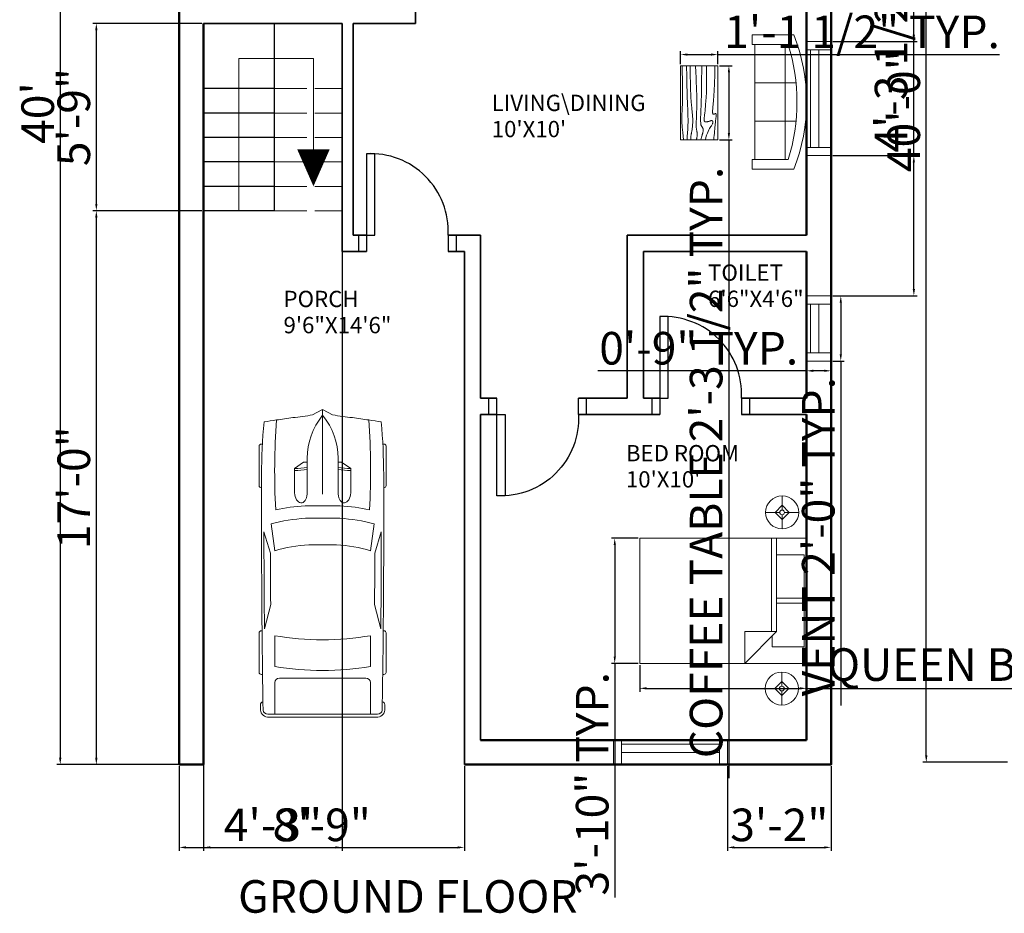
# Model space of a CAD drawing. Units: inches. Extents: x 2296 to 3335, y 495 to 1294.
# Tile 1 of 7: x 2296 to 2659, y 532 to 862. Entities that reach past the tile are written whole.
import ezdxf

# ---------------------------------------------------------------- set-up
doc = ezdxf.new("R2010")
doc.units = ezdxf.units.IN
doc.linetypes.add('ACAD_ISO02W100', pattern=[15, 12, -3])
for name, color, linetype, lineweight in [('A-ANNO-DIMS', 2, 'Continuous', 18), ('A-ANNO-SYMB', 7, 'Continuous', 18), ('A-ANNO-TEXT', 7, 'Continuous', 35), ('A-AREA-IDEN', 7, 'Continuous', 18), ('A-EQPM-VEHL', 8, 'Continuous', 13), ('A-FLOR-STRS', 7, 'Continuous', 25), ('A-FLOR-STRS-OVHD', 7, 'ACAD_ISO02W100', 18), ('DOORS', 1, 'Continuous', 25), ('E-LITE', 2, 'Continuous', 18), ('FURNITURE', 2, 'Continuous', 18), ('INNER WALL', 6, 'Continuous', 35), ('OUTER WALL', 5, 'Continuous', 50), ('VENTILATOR', 4, 'Continuous', 18), ('WINDOWS', 3, 'Continuous', 18)]:
    doc.layers.add(name, color=color, linetype=linetype, lineweight=lineweight)
doc.styles.get("Standard").update_dxf_attribs({"font": 'arial.ttf'})
doc.dimstyles.new('ISO-25', dxfattribs={"dimtxt": 12, "dimasz": 2.5, "dimexe": 1.25, "dimexo": 0.625, "dimtad": 1, "dimdec": 1, "dimlunit": 3, "dimtxsty": 'Standard', "dimcen": 2.5, "dimadec": 0, "dimazin": 0, "dimtfac": 1, "dimtdec": 1, "dimtmove": 0, "dimatfit": 3, "dimfxl": 1, "dimarcsym": 0})

# ---------------------------------------------------------------- blocks, each defined once
blk = doc.blocks.new('*U2')
for p, q in [((21.1, 37.41), (21.1, 36.83)), ((46.55, 38.89), (22.35, 38.89)), ((47.8, 37.39), (47.8, 37.41)), ((135.45, 37.07), (135.45, 37.41)), ((136.7, 38.89), (160.9, 38.89)), ((162.15, 37.41), (162.15, 36.77)), ((70.03, 31.54), (86.41, 29.35)), ((87.99, 31.87), (74.76, 35.92)), ((134.31, 35.6), (119.29, 31.78)), ((186.47, -33.5), (186.47, 33.5)), ((188.4, -32.76), (188.4, 32.76)), ((138.42, 29.35), (157.25, 29.35)), ((164.52, 26.39), (164.52, -26.39)), ((186.47, 29.35), (167.01, 29.35)), ((32.27, 11.63), (36.13, 17.17)), ((36.13, 17.17), (50.94, 17.17)), ((3.27, 6.13), (0.1, 0.41)), ((29.77, 9.51), (51.68, 9.51)), ((32.12, 9.51), (32.12, 11.15)), ((58.92, -10.77), (58.92, 10.77)), ((66.55, -10.53), (66.55, 10.53)), ((82.74, 8.5), (82.74, -8.5)), ((186.47, -10.53), (186.47, 10.53)), ((0, 0), (51.68, 0)), ((0.1, -0.41), (3.27, -6.13)), ((29.77, -9.51), (51.68, -9.51)), ((32.12, -9.51), (32.12, -11.15)), ((32.27, -11.63), (36.13, -17.17)), ((36.13, -17.17), (50.94, -17.17)), ((86.41, -29.35), (70.03, -31.54)), ((157.25, -29.35), (138.42, -29.35)), ((167.01, -29.35), (186.47, -29.35)), ((87.99, -31.87), (74.76, -35.92)), ((134.31, -35.6), (119.29, -31.78)), ((21.1, -37.41), (21.1, -36.83)), ((46.55, -38.89), (22.35, -38.89)), ((47.8, -37.39), (47.8, -37.41)), ((135.45, -37.07), (135.45, -37.41)), ((136.7, -38.89), (160.9, -38.89)), ((162.15, -37.41), (162.15, -36.77))]:
    blk.add_line(p, q)
for centre, major_axis, ratio, start_param, end_param in [((41.19, -490.86), (0, 528.23), 0.842304, 0.00281, 0.075598), ((22.35, 37.41), (0, -1.48), 0.842304, 3.141593, 4.712389), ((64.48, -10555.62), (0, 10593.03), 0.842304, -0.013397, 0.002797), ((46.55, 37.41), (0, 1.48), 0.842304, -1.570796, 0), ((136.7, 37.41), (0, -1.48), 0.842304, 3.141593, 4.712389), ((160.9, 37.41), (0, 1.48), 0.842304, -1.570796, 0), ((180.63, 35.84), (0, 2.22), 0.842304, -0.013017, 1.249894), ((64.48, -10556.36), (0, 10595.31), 0.842304, -0.013397, -0.013017), ((183.98, 33.5), (0, -2.96), 0.842304, 1.570796, 3.128196), ((183.98, 32.76), (0, -5.25), 0.842304, 1.570796, 3.128196), ((266.03, -27.52), (0, 313.31), 0.842304, 1.367076, 1.39176), ((135.29, 5.39), (0, 81.77), 0.842304, 1.245306, 1.50788), ((64.48, -10555.62), (0, -10591.55), 0.842304, 3.133765, 3.140441), ((95.79, -3666.35), (0, -3698.24), 0.842304, 3.134049, 3.144098), ((259.18, -27.52), (0, -305.3), 0.842304, 4.528606, 4.561838), ((37.47, -593.96), (0, -623.33), 0.842304, 3.096046, 3.200911), ((134.4, 5.39), (0, -89.78), 0.842304, 4.449482, 4.652344), ((149.6, 2.8), (0, -79.58), 0.842304, 4.372215, 4.640744), ((17.08, 0), (0, 147.02), 0.842304, 4.511394, 4.913384), ((35.91, 0), (0, 147.02), 0.842304, 4.511394, 4.913384), ((167.01, 26.39), (0, 2.96), 0.842304, 0, 1.570796), ((-204.49, 52.4), (0, -250.96), 0.842304, 1.385369, 1.434372), ((13.04, 17.01), (0, 27.42), 0.842304, 4.435146, 4.718221), ((14.2, 17.01), (0, 27.42), 0.842304, 4.435146, 4.718221), ((50.79, 13.34), (6.34, -0.36), 0.603834, -1.395552, 1.581315), ((29.77, -46.66), (0, 56.17), 0.842304, 0, 0.590319), ((32.75, 11.15), (0, 0.74), 0.842304, 0.879714, 1.570796), ((0.62, 0), (0, -0.74), 0.842304, 4.131459, 5.293319), ((29.77, 46.66), (0, 56.17), 0.842304, 2.551274, 3.141593), ((-204.49, -52.4), (0, 250.96), 0.842304, -1.434372, -1.385369), ((32.75, -11.15), (0, -0.74), 0.842304, 4.712389, 5.403472), ((13.04, -17.01), (0, -27.42), 0.842304, 1.564964, 1.848039), ((14.2, -17.01), (0, -27.42), 0.842304, 1.564964, 1.848039), ((134.4, -5.39), (0, -89.78), 0.842304, -1.510751, -1.307889), ((135.29, -5.39), (0, -81.77), 0.842304, -1.50788, -1.245306), ((149.6, -2.8), (0, -79.58), 0.842304, -1.499151, -1.230623), ((259.18, 27.52), (0, 305.3), 0.842304, 1.721348, 1.754579), ((266.03, 27.52), (0, 313.31), 0.842304, 1.749832, 1.774517), ((37.47, 593.96), (0, -623.33), 0.842304, -0.059319, 0.045547), ((167.01, -26.39), (0, -2.96), 0.842304, 4.712389, 6.283185), ((41.19, 490.86), (0, -528.23), 0.842304, -0.075598, -0.00281), ((64.48, 10555.62), (0, -10591.55), 0.842304, 0.001152, 0.007828), ((95.79, 3666.35), (0, -3698.24), 0.842304, -0.002505, 0.007544), ((183.98, -33.5), (0, 2.96), 0.842304, 3.15499, 4.712389), ((183.98, -32.76), (0, -5.25), 0.842304, 0.013397, 1.570796), ((22.35, -37.41), (0, 1.48), 0.842304, 1.570796, 3.141593), ((64.48, 10555.62), (0, 10593.03), 0.842304, 3.138796, 3.15499), ((46.55, -37.41), (0, -1.48), 0.842304, 0, 1.570796), ((136.7, -37.41), (0, -1.48), 0.842304, -1.570796, 0), ((160.9, -37.41), (0, 1.48), 0.842304, 3.141593, 4.712389), ((180.63, -35.84), (0, -2.22), 0.842304, -1.249894, 0.013017), ((64.48, 10556.36), (0, 10595.31), 0.842304, 3.15461, 3.15499)]:
    blk.add_ellipse(centre, major_axis=major_axis, ratio=ratio, start_param=start_param, end_param=end_param)
at = {"extrusion": (0, 0, -1)}
blk.add_ellipse((50.79, -13.34), major_axis=(6.34, 0.36), ratio=0.603834, start_param=-1.395552, end_param=1.581315, dxfattribs=at)
blk = doc.blocks.new('Sofa - Roundback 7 ft.')
for p, q in [((-36.000027, -34), (-36.000027, -11.4696)), ((-12.00002, -32.4421), (-12.00003, -6.5971)), ((11.99997, -32.4421), (11.99998, -6.5971)), ((35.99998, -34), (35.99998, -11.4696)), ((-35.999844, -13.3819), (35.9998, -13.3819)), ((-36.000027, -32.4421), (35.99998, -32.4421))]:
    blk.add_line(p, q)
for points in [[(-36.000027, -34), (-42.000027, -34), (-42.000027, -8)], [(41.99998, -8), (41.99998, -34), (35.99998, -34)]]:
    blk.add_lwpolyline(points)
for centre, radius, start, end in [((0, -114.25), 114.25, 68.43141, 111.5686), ((-0.00001, -127.1968), 121.1968, 72.72033, 107.2797)]:
    blk.add_arc(centre, radius, start, end)
blk = doc.blocks.new('Table - Rectangular Woodgrain 60 x 30 in.')
for p, q in [((0, 0), (0, -30)), ((60, 0), (0, 0)), ((60, -30), (60, 0)), ((0, -30), (60, -30))]:
    blk.add_line(p, q)
for points in [[(0, -2.4), (4.8155, -2.418), (9.0302, -2.4688), (12.709, -2.5477), (15.9167, -2.65), (18.7181, -2.7711), (21.1781, -2.9063), (23.3616, -3.0508), (25.3333, -3.2), (27.1477, -3.3495), (28.8172, -3.4958), (30.3437, -3.636), (31.7291, -3.7667), (32.9756, -3.8849), (34.0849, -3.9875), (35.059, -4.0714), (35.9, -4.1334), (36.6114, -4.1711), (37.2041, -4.1854), (37.6906, -4.1779), (38.0833, -4.15), (38.3948, -4.1034), (38.6375, -4.0396), (38.8239, -3.9602), (38.9666, -3.8667), (39.0764, -3.7608), (39.1573, -3.6448), (39.2116, -3.521), (39.2416, -3.3917), (39.2498, -3.2593), (39.2385, -3.1261), (39.21, -2.9944), (39.1666, -2.8667), (39.111, -2.7447), (39.0468, -2.6281), (38.978, -2.5163), (38.9083, -2.4083), (38.8418, -2.3035), (38.7823, -2.201), (38.7337, -2.1001), (38.7, -2), (38.6844, -1.9003), (38.6875, -1.8021), (38.7094, -1.707), (38.75, -1.6167), (38.8094, -1.5326), (38.8875, -1.4563), (38.9844, -1.3893), (39.1, -1.3333), (39.2351, -1.2896), (39.3937, -1.2583), (39.5804, -1.2396), (39.8, -1.2333), (40.057, -1.2396), (40.3562, -1.2583), (40.7023, -1.2896), (41.1, -1.3333), (41.5547, -1.3895), (42.0755, -1.4573), (42.6721, -1.5361), (43.3542, -1.625), (44.1316, -1.7233), (45.014, -1.8302), (46.0114, -1.9449), (47.1333, -2.0667), (48.3862, -2.1947), (49.7625, -2.3281), (51.2513, -2.4663), (52.8416, -2.6083), (54.5226, -2.7535), (56.2833, -2.9011), (58.1127, -3.0501), (60, -3.2)], [(0, -9.2), (6.5759, -9.0858), (11.9385, -9.0365), (16.2527, -9.0418), (19.6833, -9.0917), (22.3952, -9.1759), (24.5531, -9.2844), (26.322, -9.4069), (27.8666, -9.5333), (29.3241, -9.6553), (30.7203, -9.7719), (32.0532, -9.8837), (33.3208, -9.9917), (34.5213, -10.0965), (35.6526, -10.199), (36.7128, -10.2999), (37.7, -10.4), (38.6129, -10.4996), (39.4531, -10.5969), (40.223, -10.6895), (40.925, -10.775), (41.5613, -10.8512), (42.1344, -10.9156), (42.6465, -10.966), (43.1, -11), (43.4976, -11.0158), (43.8437, -11.0136), (44.143, -10.9942), (44.4, -10.9583), (44.6195, -10.9069), (44.8062, -10.8406), (44.9648, -10.7603), (45.1, -10.6667), (45.2155, -10.5598), (45.3114, -10.4365), (45.3871, -10.2929), (45.4416, -10.125), (45.4743, -9.929), (45.4844, -9.7011), (45.4709, -9.4371), (45.4333, -9.1333), (45.3716, -8.7883), (45.2896, -8.4104), (45.1919, -8.0107), (45.0833, -7.6), (44.9685, -7.1893), (44.8521, -6.7896), (44.7388, -6.4117), (44.6333, -6.0667), (44.54, -5.7628), (44.4614, -5.4979), (44.4001, -5.2675), (44.3583, -5.0667), (44.3384, -4.8909), (44.3427, -4.7354), (44.3736, -4.5956), (44.4333, -4.4667), (44.5236, -4.3453), (44.6427, -4.2333), (44.7884, -4.1339), (44.9583, -4.05), (45.1501, -3.9849), (45.3614, -3.9417), (45.59, -3.9234), (45.8333, -3.9333), (46.0915, -3.9749), (46.3734, -4.0531), (46.6906, -4.1736), (47.0542, -4.3417), (47.4756, -4.5629), (47.9661, -4.8427), (48.5372, -5.1866), (49.2, -5.6), (49.9676, -6.0844), (50.8594, -6.625), (51.8965, -7.2031), (53.1, -7.8), (54.491, -8.3969), (56.0906, -8.975), (57.9199, -9.5156), (60, -10)], [(0, -12.8), (5.1847, -12.9322), (9.6213, -13.0323), (13.3963, -13.1059), (16.5958, -13.1583), (19.3063, -13.1952), (21.614, -13.2219), (23.6054, -13.2439), (25.3666, -13.2667), (26.9728, -13.2947), (28.4531, -13.3281), (29.8256, -13.3663), (31.1083, -13.4083), (32.3191, -13.4535), (33.476, -13.501), (34.597, -13.5501), (35.7, -13.6), (36.7984, -13.6497), (37.8875, -13.6979), (38.9578, -13.743), (40, -13.7833), (41.0047, -13.8174), (41.9625, -13.8438), (42.864, -13.8607), (43.7, -13.8667), (44.4631, -13.8604), (45.1552, -13.8417), (45.7801, -13.8104), (46.3416, -13.7667), (46.8439, -13.7104), (47.2906, -13.6417), (47.6858, -13.5604), (48.0333, -13.4667), (48.3375, -13.3608), (48.6042, -13.2448), (48.8396, -13.121), (49.05, -12.9917), (49.2417, -12.8593), (49.4208, -12.7261), (49.5937, -12.5944), (49.7667, -12.4667), (49.9452, -12.3451), (50.1323, -12.2313), (50.3303, -12.1268), (50.5416, -12.0333), (50.7686, -11.9524), (51.0135, -11.8854), (51.2788, -11.8341), (51.5666, -11.8), (51.8785, -11.7843), (52.2116, -11.7865), (52.562, -11.8059), (52.926, -11.8417), (53.2998, -11.8931), (53.6795, -11.9594), (54.0614, -12.0397), (54.4416, -12.1333), (54.8223, -12.2401), (55.2293, -12.3625), (55.6942, -12.5037), (56.2489, -12.6667), (56.9251, -12.8547), (57.7545, -13.0708), (58.7689, -13.3182), (60, -13.6)], [(0, -18), (5.124, -17.7273), (9.6609, -17.5057), (13.6705, -17.3303), (17.2125, -17.1958), (20.3467, -17.0973), (23.1328, -17.0297), (25.6307, -16.9878), (27.9, -16.9667), (29.9928, -16.9617), (31.9302, -16.9703), (33.7254, -16.9907), (35.3917, -17.0208), (36.9423, -17.0588), (38.3906, -17.1026), (39.7499, -17.1503), (41.0333, -17.2), (42.2519, -17.2496), (43.4073, -17.2969), (44.4986, -17.3395), (45.525, -17.375), (46.4858, -17.4012), (47.3802, -17.4156), (48.2074, -17.416), (48.9667, -17.4), (49.6583, -17.3662), (50.2872, -17.3167), (50.8595, -17.2547), (51.3812, -17.1833), (51.8584, -17.1057), (52.2971, -17.025), (52.7034, -16.9443), (53.0833, -16.8667), (53.443, -16.7951), (53.789, -16.7313), (54.128, -16.6768), (54.4666, -16.6334), (54.8115, -16.6024), (55.1693, -16.5854), (55.5465, -16.5841), (55.95, -16.6), (56.3828, -16.6337), (56.8346, -16.6823), (57.2915, -16.7418), (57.7396, -16.8084), (58.165, -16.878), (58.5539, -16.9469), (58.8924, -17.0111), (59.1666, -17.0667), (59.3679, -17.1107), (59.5078, -17.1438), (59.6032, -17.1675), (59.6708, -17.1833), (59.7275, -17.193), (59.7901, -17.1979), (59.8753, -17.1998), (60, -17.2)], [(0, -22.4), (8.0098, -22.2501), (14.4094, -22.1011), (19.4168, -21.9535), (23.25, -21.8083), (26.1269, -21.6663), (28.2656, -21.5281), (29.884, -21.3947), (31.2, -21.2667), (32.3967, -21.1448), (33.5172, -21.0292), (34.5697, -20.9198), (35.5625, -20.8167), (36.5037, -20.7198), (37.4015, -20.6292), (38.2642, -20.5448), (39.1, -20.4667), (39.9164, -20.3951), (40.7187, -20.3313), (41.5117, -20.2768), (42.3, -20.2333), (43.0883, -20.2024), (43.8812, -20.1854), (44.6836, -20.1841), (45.5, -20.2), (46.3328, -20.234), (47.1747, -20.2844), (48.0163, -20.3488), (48.8479, -20.425), (49.66, -20.5106), (50.4429, -20.6031), (51.1872, -20.7004), (51.8833, -20.8), (52.5246, -20.8999), (53.1166, -20.9995), (53.6681, -21.0983), (54.1875, -21.1958), (54.6834, -21.2919), (55.1646, -21.3859), (55.6394, -21.4777), (56.1167, -21.5667), (56.6028, -21.6515), (57.0961, -21.7266), (57.5929, -21.7852), (58.0896, -21.8208), (58.5823, -21.8268), (59.0674, -21.7964), (59.5412, -21.723), (60, -21.6)], [(0, -25.2), (8.6355, -25.0504), (15.7026, -24.9031), (21.4049, -24.7606), (25.9458, -24.625), (29.529, -24.4988), (32.3578, -24.3844), (34.6359, -24.284), (36.5667, -24.2), (38.3213, -24.1341), (39.9417, -24.0854), (41.437, -24.0523), (42.8167, -24.0333), (44.0901, -24.0268), (45.2667, -24.0313), (46.3557, -24.0451), (47.3667, -24.0667), (48.309, -24.0947), (49.1928, -24.1287), (50.0284, -24.168), (50.826, -24.2125), (51.5959, -24.2617), (52.3483, -24.3151), (53.0935, -24.3725), (53.8417, -24.4334), (54.6009, -24.497), (55.3699, -24.561), (56.1454, -24.6226), (56.9239, -24.6792), (57.7021, -24.7279), (58.4764, -24.7662), (59.2435, -24.7911), (60, -24.8)], [(0, -28.8), (5.6867, -28.6681), (10.45, -28.5698), (14.407, -28.5012), (17.675, -28.4584), (20.3711, -28.4374), (22.6125, -28.4344), (24.5164, -28.4455), (26.2, -28.4667), (27.762, -28.4947), (29.2276, -28.5281), (30.6033, -28.5663), (31.8958, -28.6084), (33.1118, -28.6535), (34.2578, -28.7011), (35.3405, -28.7501), (36.3666, -28.8), (37.3443, -28.8497), (38.288, -28.8974), (39.2137, -28.9412), (40.1375, -28.9792), (41.0753, -29.0093), (42.0432, -29.0297), (43.0572, -29.0384), (44.1333, -29.0333), (45.2936, -29.0114), (46.5843, -28.9641), (48.0579, -28.8816), (49.7666, -28.7542), (51.7629, -28.5721), (54.0989, -28.3255), (56.8272, -28.0048), (60, -27.6)]]:
    blk.add_lwpolyline(points)
blk = doc.blocks.new('Bed - Queen')
for p, q in [((0, -80.00003), (0, 0)), ((0, 0), (59.99999, 0)), ((59.99999, 0), (59.99999, -80.00003)), ((7.99999, -1.2), (28.79998, -1.2)), ((7.99999, -14.4), (7.99999, -1.2)), ((28.79998, -1.2), (28.79998, -14.4)), ((31.19999, -1.2), (51.99999, -1.2)), ((31.19999, -14.4), (31.19999, -1.2)), ((51.99999, -1.2), (51.99999, -16.4)), ((0, -14.4), (44.8, -14.4)), ((44.8, -16.8), (0, -16.8)), ((59.99999, -29.6), (44.8, -14.4)), ((44.8, -14.4), (44.8, -29.6)), ((51.99999, -16.4), (46.79936, -16.4)), ((44.8, -29.6), (59.99999, -29.6)), ((59.99999, -80.00003), (0, -80.00003))]:
    blk.add_line(p, q)
blk = doc.blocks.new('Lamp - Table')
for p, q in [((0, 7), (0, 1)), ((-1, 0), (-7, 0)), ((0, 3), (-3, 0)), ((-3, 0), (0, -3)), ((3, 0), (0, 3)), ((0, -3), (3, 0)), ((1, 0), (7, 0)), ((0, -1), (0, -7))]:
    blk.add_line(p, q)
for radius in [7, 1]:
    blk.add_circle((0, 0), radius)
blk = doc.blocks.new('*D17')
at = {"layer": 'A-ANNO-DIMS', "color": 0, "lineweight": -2, "transparency": 16777216}
for p, q in [((2354.45, 1067.15), (2310.04, 1067.15)), ((2311.29, 1064.65), (2311.29, 589.65)), ((2354.45, 587.15), (2310.04, 587.15))]:
    blk.add_line(p, q, dxfattribs=at)
at = {"layer": 'A-ANNO-DIMS', "color": 0, "transparency": 16777216}
for points in [[(2310.87, 1064.65), (2311.7, 1064.65), (2311.29, 1067.15)], [(2310.87, 589.65), (2311.7, 589.65), (2311.29, 587.15)]]:
    blk.add_solid(points, dxfattribs=at)
at = {"layer": 'Defpoints', "color": 0, "transparency": 16777216}
for p in [(2355.08, 1067.15), (2311.29, 587.15), (2355.08, 587.15)]:
    blk.add_point(p, dxfattribs=at)
at = {"layer": 'A-ANNO-DIMS', "color": 0, "transparency": 16777216, "insert": (2304.54, 827.15), "char_height": 12, "attachment_point": 5, "rotation": 90}
blk.add_mtext("40'", dxfattribs=at)
blk = doc.blocks.new('DOOR-SINGLE-30IN')
for p, q in [((-3, 0), (-3, -6)), ((0, 0), (0, -6)), ((30, 0), (30, -6)), ((33, 0), (33, -6))]:
    blk.add_line(p, q)
blk.add_lwpolyline([(0, 0), (3, 0), (3, 30), (0, 30)], close=True)
blk.add_arc((1.5, 1.5), 28.54, 356.9872, 93.0128)
blk = doc.blocks.new('WIN-36IN')
for p, q in [((0, 42), (9, 42)), ((0, 39), (9, 39)), ((1.5, 3), (1.5, 39)), ((4.5, 3), (4.5, 39)), ((9, 3), (0, 3)), ((9, 0), (0, 0))]:
    blk.add_line(p, q)
blk = doc.blocks.new('VENT-18IN')
for p, q in [((0, 24), (9, 24)), ((0, 21), (9, 21)), ((4.5, 21), (4.5, 3)), ((7.5, 21), (7.5, 3)), ((9, 3), (0, 3)), ((9, 0), (0, 0))]:
    blk.add_line(p, q)
blk = doc.blocks.new('*D27')
at = {"layer": 'A-ANNO-DIMS', "color": 0, "lineweight": -2, "transparency": 16777216}
for p, q in [((2524.66, 623.83), (2524.66, 613.99)), ((2586.06, 623.83), (2586.06, 613.99)), ((2527.16, 615.24), (2583.56, 615.24)), ((2586.06, 615.24), (2794.3, 615.24))]:
    blk.add_line(p, q, dxfattribs=at)
at = {"layer": 'A-ANNO-DIMS', "color": 0, "transparency": 16777216}
for points in [[(2527.16, 615.66), (2527.16, 614.82), (2524.66, 615.24)], [(2583.56, 615.66), (2583.56, 614.82), (2586.06, 615.24)]]:
    blk.add_solid(points, dxfattribs=at)
at = {"layer": 'Defpoints', "color": 0, "transparency": 16777216}
for p in [(2524.66, 624.45), (2586.06, 624.45), (2586.06, 615.24)]:
    blk.add_point(p, dxfattribs=at)
at = {"layer": 'A-ANNO-DIMS', "color": 0, "transparency": 16777216, "insert": (2691.43, 622.44), "char_height": 12, "attachment_point": 5}
blk.add_mtext('QUEEN BED 5\'-1 1/2" TYP.', dxfattribs=at)
blk = doc.blocks.new('*D28')
at = {"layer": 'A-ANNO-DIMS', "color": 0, "lineweight": -2, "transparency": 16777216}
for p, q in [((2524.04, 670.5), (2514.2, 670.5)), ((2515.45, 668), (2515.45, 626.95)), ((2524.04, 624.45), (2514.2, 624.45)), ((2515.45, 624.45), (2515.45, 538.24))]:
    blk.add_line(p, q, dxfattribs=at)
at = {"layer": 'A-ANNO-DIMS', "color": 0, "transparency": 16777216}
for points in [[(2515.04, 668), (2515.87, 668), (2515.45, 670.5)], [(2515.04, 626.95), (2515.87, 626.95), (2515.45, 624.45)]]:
    blk.add_solid(points, dxfattribs=at)
at = {"layer": 'Defpoints', "color": 0, "transparency": 16777216}
for p in [(2524.66, 670.5), (2515.45, 624.45), (2524.66, 624.45)]:
    blk.add_point(p, dxfattribs=at)
at = {"layer": 'A-ANNO-DIMS', "color": 0, "transparency": 16777216, "insert": (2508.7, 580.09), "char_height": 12, "attachment_point": 5, "rotation": 90}
blk.add_mtext('3\'-10" TYP.', dxfattribs=at)
blk = doc.blocks.new('*D33')
at = {"layer": 'A-ANNO-DIMS', "color": 0, "lineweight": -2, "transparency": 16777216}
for p, q in [((2595.7, 759.8), (2599.93, 759.8)), ((2598.68, 757.3), (2598.68, 738.3)), ((2595.7, 735.8), (2599.93, 735.8)), ((2598.68, 735.8), (2598.68, 608.92))]:
    blk.add_line(p, q, dxfattribs=at)
at = {"layer": 'A-ANNO-DIMS', "color": 0, "transparency": 16777216}
for points in [[(2598.26, 757.3), (2599.09, 757.3), (2598.68, 759.8)], [(2598.26, 738.3), (2599.09, 738.3), (2598.68, 735.8)]]:
    blk.add_solid(points, dxfattribs=at)
at = {"layer": 'Defpoints', "color": 0, "transparency": 16777216}
for p in [(2595.08, 759.8), (2595.08, 735.8), (2598.68, 735.8)]:
    blk.add_point(p, dxfattribs=at)
at = {"layer": 'A-ANNO-DIMS', "color": 0, "transparency": 16777216, "insert": (2591.93, 671.11), "char_height": 12, "attachment_point": 5, "rotation": 90}
blk.add_mtext('VENT 2\'-0" TYP.', dxfattribs=at)
blk = doc.blocks.new('*D34')
at = {"layer": 'A-ANNO-DIMS', "color": 0, "lineweight": -2, "transparency": 16777216}
for p, q in [((2586.08, 735.18), (2586.08, 730.95)), ((2595.08, 735.18), (2595.08, 730.95)), ((2586.08, 732.2), (2509.18, 732.2)), ((2592.58, 732.2), (2588.58, 732.2))]:
    blk.add_line(p, q, dxfattribs=at)
at = {"layer": 'A-ANNO-DIMS', "color": 0, "transparency": 16777216}
for points in [[(2588.58, 732.62), (2588.58, 731.79), (2586.08, 732.2)], [(2592.58, 732.62), (2592.58, 731.79), (2595.08, 732.2)]]:
    blk.add_solid(points, dxfattribs=at)
at = {"layer": 'Defpoints', "color": 0, "transparency": 16777216}
for p in [(2586.08, 735.8), (2595.08, 735.8), (2586.08, 732.2)]:
    blk.add_point(p, dxfattribs=at)
at = {"layer": 'A-ANNO-DIMS', "color": 0, "transparency": 16777216, "insert": (2546.38, 738.96), "char_height": 12, "attachment_point": 5}
blk.add_mtext('0\'-9" TYP.', dxfattribs=at)
blk = doc.blocks.new('*D45')
at = {"layer": 'A-ANNO-DIMS', "color": 0, "lineweight": -2, "transparency": 16777216}
for p, q in [((2554.01, 844.58), (2558.73, 844.58)), ((2557.48, 842.08), (2557.48, 819.74)), ((2554.01, 817.24), (2558.73, 817.24)), ((2557.48, 817.24), (2557.48, 582.11))]:
    blk.add_line(p, q, dxfattribs=at)
at = {"layer": 'A-ANNO-DIMS', "color": 0, "transparency": 16777216}
for points in [[(2557.07, 842.08), (2557.9, 842.08), (2557.48, 844.58)], [(2557.07, 819.74), (2557.9, 819.74), (2557.48, 817.24)]]:
    blk.add_solid(points, dxfattribs=at)
at = {"layer": 'Defpoints', "color": 0, "transparency": 16777216}
for p in [(2553.38, 844.58), (2553.38, 817.24), (2557.48, 817.24)]:
    blk.add_point(p, dxfattribs=at)
at = {"layer": 'A-ANNO-DIMS', "color": 0, "transparency": 16777216, "insert": (2550.65, 698.43), "char_height": 12, "attachment_point": 5, "rotation": 90}
blk.add_mtext('COFFEE TABLE 2\'-3 1/2" TYP.', dxfattribs=at)
blk = doc.blocks.new('*D46')
at = {"layer": 'A-ANNO-DIMS', "color": 0, "lineweight": -2, "transparency": 16777216}
for p, q in [((2539.71, 845.21), (2539.71, 849.93)), ((2542.21, 848.68), (2550.88, 848.68)), ((2553.38, 845.21), (2553.38, 849.93)), ((2553.38, 848.68), (2657.11, 848.68))]:
    blk.add_line(p, q, dxfattribs=at)
at = {"layer": 'A-ANNO-DIMS', "color": 0, "transparency": 16777216}
for points in [[(2542.21, 849.1), (2542.21, 848.27), (2539.71, 848.68)], [(2550.88, 849.1), (2550.88, 848.27), (2553.38, 848.68)]]:
    blk.add_solid(points, dxfattribs=at)
at = {"layer": 'Defpoints', "color": 0, "transparency": 16777216}
for p in [(2553.38, 848.68), (2539.71, 844.58), (2553.38, 844.58)]:
    blk.add_point(p, dxfattribs=at)
at = {"layer": 'A-ANNO-DIMS', "color": 0, "transparency": 16777216, "insert": (2606.5, 855.51), "char_height": 12, "attachment_point": 5}
blk.add_mtext('1\'-1 1/2" TYP.', dxfattribs=at)
blk = doc.blocks.new('*D52')
at = {"layer": 'A-ANNO-DIMS', "color": 0, "lineweight": -2, "transparency": 16777216}
for p, q in [((2660.03, 1068.02), (2628.91, 1068.02)), ((2630.16, 590.52), (2630.16, 1065.52)), ((2660.03, 588.02), (2628.91, 588.02))]:
    blk.add_line(p, q, dxfattribs=at)
at = {"layer": 'A-ANNO-DIMS', "color": 0, "transparency": 16777216}
for points in [[(2629.74, 1065.52), (2630.57, 1065.52), (2630.16, 1068.02)], [(2629.74, 590.52), (2630.57, 590.52), (2630.16, 588.02)]]:
    blk.add_solid(points, dxfattribs=at)
at = {"layer": 'Defpoints', "color": 0, "transparency": 16777216}
for p in [(2630.16, 1068.02), (2660.66, 1068.02), (2660.66, 588.02)]:
    blk.add_point(p, dxfattribs=at)
at = {"layer": 'A-ANNO-DIMS', "color": 0, "transparency": 16777216, "insert": (2623.41, 828.02), "char_height": 12, "attachment_point": 5, "rotation": 90}
blk.add_mtext('40\'-0"', dxfattribs=at)
blk = doc.blocks.new('*D56')
at = {"layer": 'A-ANNO-DIMS', "color": 0, "lineweight": -2, "transparency": 16777216}
for p, q in [((2595.7, 954.3), (2626.83, 954.3)), ((2625.58, 855.97), (2625.58, 951.8)), ((2595.7, 853.47), (2626.83, 853.47))]:
    blk.add_line(p, q, dxfattribs=at)
at = {"layer": 'A-ANNO-DIMS', "color": 0, "transparency": 16777216}
for points in [[(2625.16, 951.8), (2625.99, 951.8), (2625.58, 954.3)], [(2625.16, 855.97), (2625.99, 855.97), (2625.58, 853.47)]]:
    blk.add_solid(points, dxfattribs=at)
at = {"layer": 'Defpoints', "color": 0, "transparency": 16777216}
for p in [(2595.08, 954.3), (2625.58, 954.3), (2595.08, 853.47)]:
    blk.add_point(p, dxfattribs=at)
at = {"layer": 'A-ANNO-DIMS', "color": 0, "transparency": 16777216, "insert": (2618.83, 903.89), "char_height": 12, "attachment_point": 5, "rotation": 90}
blk.add_mtext('8\'-5"', dxfattribs=at)
blk = doc.blocks.new('*D57')
at = {"layer": 'A-ANNO-DIMS', "color": 0, "lineweight": -2, "transparency": 16777216}
for p, q in [((2625.58, 811.47), (2625.58, 875.57)), ((2595.7, 811.47), (2626.83, 811.47)), ((2625.58, 762.3), (2625.58, 808.97)), ((2595.7, 759.8), (2626.83, 759.8))]:
    blk.add_line(p, q, dxfattribs=at)
at = {"layer": 'A-ANNO-DIMS', "color": 0, "transparency": 16777216}
for points in [[(2625.16, 808.97), (2625.99, 808.97), (2625.58, 811.47)], [(2625.16, 762.3), (2625.99, 762.3), (2625.58, 759.8)]]:
    blk.add_solid(points, dxfattribs=at)
at = {"layer": 'Defpoints', "color": 0, "transparency": 16777216}
for p in [(2595.08, 811.47), (2625.58, 811.47), (2595.08, 759.8)]:
    blk.add_point(p, dxfattribs=at)
at = {"layer": 'A-ANNO-DIMS', "color": 0, "transparency": 16777216, "insert": (2618.74, 844.77), "char_height": 12, "attachment_point": 5, "rotation": 90}
blk.add_mtext('4\'-3 1/2"', dxfattribs=at)
blk = doc.blocks.new('*D59')
at = {"layer": 'A-ANNO-DIMS', "color": 0, "lineweight": -2, "transparency": 16777216}
for p, q in [((2556.99, 586.52), (2556.99, 555.4)), ((2595.08, 586.52), (2595.08, 555.4)), ((2559.49, 556.65), (2592.58, 556.65))]:
    blk.add_line(p, q, dxfattribs=at)
at = {"layer": 'A-ANNO-DIMS', "color": 0, "transparency": 16777216}
for points in [[(2559.49, 557.06), (2559.49, 556.23), (2556.99, 556.65)], [(2592.58, 557.06), (2592.58, 556.23), (2595.08, 556.65)]]:
    blk.add_solid(points, dxfattribs=at)
at = {"layer": 'Defpoints', "color": 0, "transparency": 16777216}
for p in [(2556.99, 587.15), (2595.08, 587.15), (2595.08, 556.65)]:
    blk.add_point(p, dxfattribs=at)
at = {"layer": 'A-ANNO-DIMS', "color": 0, "transparency": 16777216, "insert": (2576.04, 563.4), "char_height": 12, "attachment_point": 5}
blk.add_mtext('3\'-2"', dxfattribs=at)
blk = doc.blocks.new('*D60')
at = {"layer": 'A-ANNO-DIMS', "color": 0, "lineweight": -2, "transparency": 16777216}
for p, q in [((2355.08, 586.52), (2355.08, 555.4)), ((2460.08, 586.52), (2460.08, 555.4)), ((2357.58, 556.65), (2457.58, 556.65))]:
    blk.add_line(p, q, dxfattribs=at)
at = {"layer": 'A-ANNO-DIMS', "color": 0, "transparency": 16777216}
for points in [[(2357.58, 557.06), (2357.58, 556.23), (2355.08, 556.65)], [(2457.58, 557.06), (2457.58, 556.23), (2460.08, 556.65)]]:
    blk.add_solid(points, dxfattribs=at)
at = {"layer": 'Defpoints', "color": 0, "transparency": 16777216}
for p in [(2355.08, 587.15), (2460.08, 587.15), (2460.08, 556.65)]:
    blk.add_point(p, dxfattribs=at)
at = {"layer": 'A-ANNO-DIMS', "color": 0, "transparency": 16777216, "insert": (2407.58, 563.4), "char_height": 12, "attachment_point": 5}
blk.add_mtext('8\'-9"', dxfattribs=at)
blk = doc.blocks.new('*D61')
at = {"layer": 'A-ANNO-DIMS', "color": 0, "lineweight": -2, "transparency": 16777216}
for p, q in [((2364.08, 790.52), (2364.08, 555.4)), ((2415.08, 790.52), (2415.08, 555.4)), ((2366.58, 556.65), (2412.58, 556.65))]:
    blk.add_line(p, q, dxfattribs=at)
at = {"layer": 'A-ANNO-DIMS', "color": 0, "transparency": 16777216}
for points in [[(2366.58, 557.06), (2366.58, 556.23), (2364.08, 556.65)], [(2412.58, 557.06), (2412.58, 556.23), (2415.08, 556.65)]]:
    blk.add_solid(points, dxfattribs=at)
at = {"layer": 'Defpoints', "color": 0, "transparency": 16777216}
for p in [(2364.08, 791.15), (2415.08, 791.15), (2415.08, 556.65)]:
    blk.add_point(p, dxfattribs=at)
at = {"layer": 'A-ANNO-DIMS', "color": 0, "transparency": 16777216, "insert": (2389.58, 563.4), "char_height": 12, "attachment_point": 5}
blk.add_mtext('4\'-3"', dxfattribs=at)
blk = doc.blocks.new('*D62')
at = {"layer": 'A-ANNO-DIMS', "color": 0, "lineweight": -2, "transparency": 16777216}
for p, q in [((2363.45, 791.15), (2323.33, 791.15)), ((2324.58, 589.65), (2324.58, 788.65)), ((2363.45, 587.15), (2323.33, 587.15))]:
    blk.add_line(p, q, dxfattribs=at)
at = {"layer": 'A-ANNO-DIMS', "color": 0, "transparency": 16777216}
for points in [[(2324.16, 788.65), (2324.99, 788.65), (2324.58, 791.15)], [(2324.16, 589.65), (2324.99, 589.65), (2324.58, 587.15)]]:
    blk.add_solid(points, dxfattribs=at)
at = {"layer": 'Defpoints', "color": 0, "transparency": 16777216}
for p in [(2324.58, 791.15), (2364.08, 791.15), (2364.08, 587.15)]:
    blk.add_point(p, dxfattribs=at)
at = {"layer": 'A-ANNO-DIMS', "color": 0, "transparency": 16777216, "insert": (2317.83, 689.15), "char_height": 12, "attachment_point": 5, "rotation": 90}
blk.add_mtext('17\'-0"', dxfattribs=at)
blk = doc.blocks.new('*D63')
at = {"layer": 'A-ANNO-DIMS', "color": 0, "lineweight": -2, "transparency": 16777216}
for p, q in [((2363.45, 860.15), (2323.33, 860.15)), ((2324.58, 793.65), (2324.58, 857.65)), ((2363.45, 791.15), (2323.33, 791.15))]:
    blk.add_line(p, q, dxfattribs=at)
at = {"layer": 'A-ANNO-DIMS', "color": 0, "transparency": 16777216}
for points in [[(2324.16, 857.65), (2324.99, 857.65), (2324.58, 860.15)], [(2324.16, 793.65), (2324.99, 793.65), (2324.58, 791.15)]]:
    blk.add_solid(points, dxfattribs=at)
at = {"layer": 'Defpoints', "color": 0, "transparency": 16777216}
for p in [(2324.58, 860.15), (2364.08, 860.15), (2364.08, 791.15)]:
    blk.add_point(p, dxfattribs=at)
at = {"layer": 'A-ANNO-DIMS', "color": 0, "transparency": 16777216, "insert": (2317.83, 825.65), "char_height": 12, "attachment_point": 5, "rotation": 90}
blk.add_mtext('5\'-9"', dxfattribs=at)

msp = doc.modelspace()

# ---------------------------------------------------------------- linework, layer by layer
at = {"layer": 'A-ANNO-SYMB'}
msp.add_lwpolyline([(2377.08, 791.15), (2377.08, 847.25), (2404.52, 847.25), (2404.52, 813.81)], dxfattribs=at)
msp.add_lwpolyline([(2404.52, 813.81, 12, 0, 0), (2404.52, 800.15, 0, 0, 0)], format="xyseb", dxfattribs=at)
at = {"layer": 'A-FLOR-STRS'}
for p, q in [((2390.08, 860.15), (2390.08, 791.15)), ((2390.08, 836.15), (2364.08, 836.15)), ((2390.08, 827.15), (2364.08, 827.15)), ((2390.08, 818.15), (2364.08, 818.15)), ((2390.08, 809.15), (2364.08, 809.15)), ((2390.08, 800.15), (2364.08, 800.15)), ((2390.08, 791.15), (2364.08, 791.15))]:
    msp.add_line(p, q, dxfattribs=at)
at = {"layer": 'A-FLOR-STRS-OVHD'}
for p, q in [((2390.08, 836.15), (2415.08, 836.15)), ((2390.08, 827.15), (2415.08, 827.15)), ((2390.08, 818.15), (2415.08, 818.15)), ((2390.08, 809.15), (2415.08, 809.15)), ((2390.08, 800.15), (2415.08, 800.15)), ((2390.08, 791.15), (2415.08, 791.15))]:
    msp.add_line(p, q, dxfattribs=at)
at = {"layer": 'INNER WALL'}
for p, q in [((2442.08, 914.15), (2442.08, 860.15)), ((2415.08, 860.15), (2364.08, 860.15)), ((2415.08, 860.15), (2415.08, 776.15)), ((2442.08, 860.15), (2419.08, 860.15)), ((2419.08, 860.15), (2419.08, 782.15)), ((2419.08, 782.15), (2424.08, 782.15)), ((2454.08, 782.15), (2466.08, 782.15)), ((2466.08, 722.15), (2466.08, 782.15)), ((2520.08, 782.15), (2586.08, 782.15)), ((2520.08, 722.15), (2520.08, 782.15)), ((2415.08, 776.15), (2424.08, 776.15)), ((2454.08, 776.15), (2460.08, 776.15)), ((2460.08, 587.15), (2460.08, 776.15)), ((2526.08, 722.15), (2526.08, 776.15)), ((2526.08, 776.15), (2586.08, 776.15)), ((2466.08, 722.15), (2472.08, 722.15)), ((2502.08, 722.15), (2520.08, 722.15)), ((2526.08, 722.15), (2532.08, 722.15)), ((2562.08, 722.15), (2586.08, 722.15)), ((2466.08, 716.15), (2472.08, 716.15)), ((2466.08, 596.15), (2466.08, 716.15)), ((2502.08, 716.15), (2532.08, 716.15)), ((2562.08, 716.15), (2586.08, 716.15))]:
    msp.add_line(p, q, dxfattribs=at)
at = {"layer": 'OUTER WALL'}
for p, q in [((2586.08, 782.15), (2586.08, 884.15)), ((2364.08, 860.15), (2364.08, 776.15)), ((2364.08, 776.15), (2364.08, 587.15)), ((2586.08, 722.15), (2586.08, 776.15)), ((2586.08, 596.15), (2586.08, 716.15)), ((2466.08, 596.15), (2586.08, 596.15))]:
    msp.add_line(p, q, dxfattribs=at)
msp.add_lwpolyline([(2460.08, 587.15), (2595.08, 587.15), (2595.08, 1067.15), (2355.08, 1067.15), (2355.08, 587.15), (2364.08, 587.15)], dxfattribs=at)

# ---------------------------------------------------------------- block references
at = {"layer": 'A-EQPM-VEHL', "xscale": 0.6015858060565531, "yscale": 0.6015858060565531, "zscale": 0.6015858060565531, "rotation": 270}
msp.add_blockref('*U2', (2407.9, 717.91), dxfattribs=at)
at = {"layer": 'DOORS'}
for p in [(2424.08, 782.15), (2532.08, 722.15)]:
    msp.add_blockref('DOOR-SINGLE-30IN', p, dxfattribs=at)
at = {"layer": 'DOORS', "extrusion": (0, 0, -1), "zscale": -1, "rotation": 180}
msp.add_blockref('DOOR-SINGLE-30IN', (-2472.08, 716.15), dxfattribs=at)
at = {"layer": 'E-LITE', "xscale": 0.8700180084150424, "yscale": 0.8700180084150424, "zscale": 0.8700180084150424}
for p in [(2577.09, 680.05), (2576.97, 615.16)]:
    msp.add_blockref('Lamp - Table', p, dxfattribs=at)
at = {"layer": 'FURNITURE', "rotation": 270}
for name, p, xscale, yscale, zscale in [('Sofa - Roundback 7 ft.', (2586.08, 831.2), 0.588291610216848, 0.588291610216848, 0.588291610216848), ('Table - Rectangular Woodgrain 60 x 30 in.', (2553.38, 844.58), 0.455660307090303, 0.455660307090303, 0.455660307090303), ('Bed - Queen', (2586.06, 670.5), 0.7674836837443932, 0.7674836837443932, 0.7674836837443932)]:
    msp.add_blockref(name, p, dxfattribs=dict(at, xscale=xscale, yscale=yscale, zscale=zscale))
at = {"layer": 'VENTILATOR', "rotation": 180}
msp.add_blockref('VENT-18IN', (2595.08, 759.8), dxfattribs=at)
at = {"layer": 'WINDOWS'}
msp.add_blockref('WIN-36IN', (2586.08, 811.47), dxfattribs=at)
at = {"layer": 'WINDOWS', "rotation": 269.9999999999991}
msp.add_blockref('WIN-36IN', (2514.99, 596.15), dxfattribs=at)

# ---------------------------------------------------------------- texts
at = {"layer": 'A-ANNO-TEXT'}
msp.add_text('GROUND FLOOR', height=12, dxfattribs=at).set_placement((2376.77, 532.59))
at = {"layer": 'A-AREA-IDEN'}
for s, p in [('LIVING\\DINING', (2470.16, 827.89)), ("10'X10'", (2470.16, 818.25)), ('TOILET', (2549.82, 765.36)), ('PORCH', (2393.5, 755.67)), ('6\'6"X4\'6"', (2549.82, 755.72)), ('9\'6"X14\'6"', (2393.5, 746.03)), ('BED ROOM', (2519.57, 698.86)), ("10'X10'", (2519.57, 689.22))]:
    msp.add_text(s, height=6, dxfattribs=at).set_placement(p)

# ---------------------------------------------------------------- dimensions: what is measured, and where the dimension line sits
at = {"layer": 'A-ANNO-DIMS'}
for base, p1, p2, override, picture, middle in [((2311.29, 587.15), (2355.08, 1067.15), (2355.08, 587.15), {"dimclrd": 0, "dimclre": 0, "dimclrt": 0}, '*D17', (2304.54, 827.15)), ((2630.16, 1068.02), (2660.66, 588.02), (2660.66, 1068.02), {"dimdec": 1, "dimlfac": 1, "dimrnd": 0, "dimzin": 1, "dimdsep": 46, "dimlunit": 4, "dimfrac": 2}, '*D52', (2623.41, 828.02)), ((2625.58, 954.3), (2595.08, 853.47), (2595.08, 954.3), {"dimdec": 1, "dimlfac": 1, "dimrnd": 0, "dimzin": 1, "dimdsep": 46, "dimlunit": 4, "dimfrac": 2}, '*D56', (2618.83, 903.89)), ((2625.58, 811.47), (2595.08, 759.8), (2595.08, 811.47), {"dimdec": 1, "dimlfac": 1, "dimrnd": 0, "dimzin": 1, "dimdsep": 46, "dimlunit": 4, "dimfrac": 2}, '*D57', (2618.74, 844.77)), ((2324.58, 860.15), (2364.08, 791.15), (2364.08, 860.15), {"dimdec": 1, "dimlfac": 1, "dimrnd": 0, "dimzin": 1, "dimdsep": 46, "dimlunit": 4, "dimfrac": 2}, '*D63', (2317.83, 825.65)), ((2324.58, 791.15), (2364.08, 587.15), (2364.08, 791.15), {"dimdec": 1, "dimlfac": 1, "dimrnd": 0, "dimzin": 1, "dimdsep": 46, "dimlunit": 4, "dimfrac": 2}, '*D62', (2317.83, 689.15))]:
    dim = msp.add_linear_dim(base=base, p1=p1, p2=p2, angle=90, dimstyle='ISO-25', override=override, dxfattribs=at)
    dim.commit()
    dim.dimension.update_dxf_attribs({"geometry": picture, "text_midpoint": middle})
for base, p1, p2, text, picture, middle in [((2553.38, 848.68), (2539.71, 844.58), (2553.38, 844.58), '<> TYP.', '*D46', (2606.5, 855.51)), ((2586.06, 615.24), (2524.66, 624.45), (2586.06, 624.45), 'QUEEN BED <> TYP.', '*D27', (2691.43, 622.44))]:
    dim = msp.add_linear_dim(base=base, p1=p1, p2=p2, text=text, dimstyle='ISO-25', override={"dimdec": 1, "dimlfac": 1, "dimrnd": 0, "dimzin": 1, "dimdsep": 46, "dimlunit": 4, "dimfrac": 2}, dxfattribs=at)
    dim.commit()
    dim.dimension.update_dxf_attribs({"geometry": picture, "text_midpoint": middle})
for base, p1, p2, angle, text, picture, middle in [((2557.48, 817.24), (2553.38, 844.58), (2553.38, 817.24), 270, 'COFFEE TABLE <> TYP.', '*D45', (2550.65, 698.43)), ((2598.68, 735.8), (2595.08, 759.8), (2595.08, 735.8), 270, 'VENT <> TYP.', '*D33', (2591.93, 671.11)), ((2586.08, 732.2), (2595.08, 735.8), (2586.08, 735.8), 180, '<> TYP.', '*D34', (2546.38, 738.96)), ((2515.4542, 624.4501), (2524.664, 670.4991), (2524.664, 624.4501), 270, '<> TYP.', '*D28', (2508.6982, 580.0945))]:
    dim = msp.add_linear_dim(base=base, p1=p1, p2=p2, angle=angle, text=text, dimstyle='ISO-25', override={"dimdec": 1, "dimlfac": 1, "dimrnd": 0, "dimzin": 1, "dimdsep": 46, "dimlunit": 4, "dimfrac": 2}, dxfattribs=at)
    dim.commit()
    dim.dimension.update_dxf_attribs({"geometry": picture, "text_midpoint": middle})
for base, p1, p2, picture, middle in [((2415.08, 556.65), (2364.08, 791.15), (2415.08, 791.15), '*D61', (2389.58, 563.4)), ((2460.08, 556.65), (2355.08, 587.15), (2460.08, 587.15), '*D60', (2407.58, 563.4)), ((2595.08, 556.65), (2556.99, 587.15), (2595.08, 587.15), '*D59', (2576.04, 563.4))]:
    dim = msp.add_linear_dim(base=base, p1=p1, p2=p2, dimstyle='ISO-25', override={"dimdec": 1, "dimlfac": 1, "dimrnd": 0, "dimzin": 1, "dimdsep": 46, "dimlunit": 4, "dimfrac": 2}, dxfattribs=at)
    dim.commit()
    dim.dimension.update_dxf_attribs({"geometry": picture, "text_midpoint": middle})

doc.saveas('drawing.dxf')
